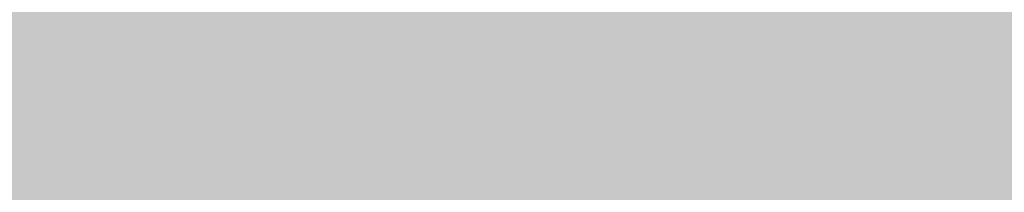
# Model space of a CAD drawing. Units: inches. Extents: x 2091 to 2899, y 967 to 2217.
# Tile 218 of 256: x 2203.2571 to 2203.4104, y 1152.274 to 1152.3009. Entities that reach past the tile are written whole.
import ezdxf

# ---------------------------------------------------------------- set-up
doc = ezdxf.new("R2010")
doc.units = ezdxf.units.IN
doc.layers.add('A-WALL-PATT', color=141, linetype='Continuous', lineweight=13, true_color=0xadddf7)

msp = doc.modelspace()

# ---------------------------------------------------------------- hatches: boundary and pattern name
at = {"layer": 'A-WALL-PATT'}
h = msp.add_hatch(color=256, dxfattribs=at)
h.dxf.hatch_style = 1
h.paths.add_polyline_path([(2803.1436, 2050.91906), (2203.1436, 2050.91906), (2203.1436, 1090.91906), (2803.1436, 1090.91906)])
h.paths.add_polyline_path([(2635.79885, 1147.54046), (2674.52405, 1147.54046, 0.376086), (2678.52967, 1152.8802), (2678.52967, 1159.55647, 0.333335), (2674.52432, 1163.56185), (2674.52432, 1163.56185), (2674.52432, 1192.93439), (2635.80597, 1192.93439), (2597.08762, 1192.93439), (2597.08762, 1163.56185, 0.333335), (2593.08228, 1159.55647), (2593.08228, 1152.8802, 0.376086), (2597.08789, 1147.54046)], flags=0)
h.paths.add_polyline_path([(2436.01043, 1278.24078, 0.000483), (2435.95264, 1278.21503, -0.001328), (2435.93563, 1278.11169, -0.001711), (2436.11644, 1278.04076, 0.002185)], flags=0)
h.paths.add_polyline_path([(2794.1436, 1143.41906), (2794.1436, 1347.41906), (2543.37017, 1347.41906), (2543.37017, 1351.91906), (2794.1436, 1351.91906), (2794.1436, 1392.71355), (2793.9474, 1392.71355), (2793.9474, 1473.5369), (2794.1436, 1473.5369), (2794.1436, 1531.91906), (2650.1436, 1531.91906), (2650.1436, 1536.41906), (2794.1436, 1536.41906), (2794.1436, 1692.41906), (2609.37561, 1692.41906), (2609.37561, 1644.41906), (2604.87561, 1644.41906), (2604.87561, 1744.91906), (2609.37561, 1744.91906), (2609.37561, 1696.91906), (2794.1436, 1696.91906), (2794.1436, 1780.91906), (2609.6436, 1780.91906), (2493.87561, 1780.91906), (2493.87561, 1785.41906), (2609.6436, 1785.41906), (2794.1436, 1785.41906), (2794.1436, 1847.93882), (2793.95122, 1847.93882), (2793.95122, 1928.76217), (2794.1436, 1928.76217), (2794.1436, 1941.41906), (2614.1436, 1941.41906), (2614.1436, 1821.41906), (2609.6436, 1821.41906), (2609.6436, 1941.41906), (2392.1436, 1941.41906), (2392.1436, 1819.91906), (2387.6436, 1819.91906), (2387.6436, 1941.41906), (2212.1436, 1941.41906), (2212.1436, 1783.91906), (2392.1436, 1783.91906), (2392.1436, 1780.91906), (2212.1436, 1780.91906), (2212.1436, 1629.41906), (2387.6436, 1629.41906), (2387.6436, 1744.91906), (2392.1436, 1744.91906), (2392.1436, 1627.91906), (2317.1436, 1627.91906), (2317.1436, 1551.41906), (2317.1436, 1536.41906), (2459.38359, 1536.41906), (2459.38359, 1602.39648), (2463.88359, 1602.39648), (2463.88359, 1531.91906), (2456.6436, 1531.91906), (2456.6436, 1529.91906), (2452.1436, 1529.91906), (2452.1436, 1531.91906), (2312.6436, 1531.91906), (2312.6436, 1551.41906), (2306.1436, 1551.41906), (2306.1436, 1555.91906), (2308.1436, 1555.91906), (2308.1436, 1551.41906), (2312.6436, 1551.41906), (2312.6436, 1627.91906), (2212.1436, 1627.91906), (2212.1436, 1555.91906), (2270.1436, 1555.91906), (2270.1436, 1551.41906), (2212.1436, 1551.41906), (2212.1436, 1351.91906), (2272.1436, 1351.91906), (2272.1436, 1347.41906), (2212.1436, 1347.41906), (2212.1436, 1275.41906), (2308.1436, 1275.41906), (2308.1436, 1351.91906), (2452.1436, 1351.91906), (2452.1436, 1493.91906), (2456.6436, 1493.91906), (2456.6436, 1347.41906), (2312.6436, 1347.41906), (2312.6436, 1270.91906), (2212.1436, 1270.91906), (2212.1436, 1099.91906), (2281.23752, 1099.91906), (2282.87104, 1110.9138), (2282.00834, 1116.9966), (2278.55774, 1121.4204), (2268.20564, 1128.0562), (2272.08764, 1128.0562), (2273.81294, 1131.927), (2279.42034, 1134.6919), (2285.02784, 1135.2449), (2287.61584, 1137.4568), (2288.04714, 1138.0098), (2289.34114, 1140.7747), (2291.06654, 1139.6687), (2292.36054, 1135.2449), (2295.37984, 1136.9038), (2296.24254, 1135.7979), (2297.10524, 1133.033), (2300.12464, 1138.0098), (2303.14394, 1138.0098), (2304.43794, 1135.7979), (2303.14394, 1133.586), (2306.59464, 1134.6919), (2307.88874, 1133.033), (2310.90804, 1135.2449), (2313.92744, 1134.1389), (2315.62686, 1132.4271), (2308.32004, 1117.5496), (2290.20384, 1109.8079), (2288.90984, 1103.1721), (2289.27231, 1099.91906), (2434.91823, 1099.91906), (2431.59323, 1124.78806), (2429.93023, 1169.55306), (2430.92718, 1240.51969), (2435.65893, 1238.18613), (2437.13523, 1196.55406), (2438.79823, 1143.97306), (2442.67823, 1111.99806), (2446.55823, 1099.91906), (2794.1436, 1099.91906), (2794.1436, 1138.91906), (2548.03245, 1138.91906), (2548.03245, 1143.41906), (2548.03245, 1148.81906), (2546.66846, 1148.03156), (2528.68569, 1179.17862, 0.256256), (2512.03245, 1148.81906), (2512.03245, 1143.41906), (2512.03245, 1138.91906), (2507.53245, 1138.91906), (2507.53245, 1143.41906), (2507.53245, 1148.81906, 0.256256), (2490.8792, 1179.17862), (2472.89644, 1148.03156), (2471.53245, 1148.81906), (2471.53245, 1143.41906), (2467.03245, 1143.41906), (2467.03245, 1269.94579, 0.039061), (2460.90999, 1273.58006), (2467.03245, 1273.58006), (2467.03245, 1286.32536, 0.014511), (2465.21619, 1286.76191), (2467.03245, 1287.05258), (2467.03245, 1323.41906), (2471.53245, 1323.41906), (2471.53245, 1148.81906), (2489.53245, 1179.99597), (2490.89644, 1179.20847), (2490.8792, 1179.17862, -0.256256), (2507.53245, 1148.81906), (2507.53245, 1143.41906), (2512.03245, 1143.41906), (2512.03245, 1148.81906, -0.256256), (2528.68569, 1179.17862), (2528.66846, 1179.20847), (2530.03245, 1179.99597), (2548.03245, 1148.81906), (2548.03245, 1143.41906)], flags=16)
h.paths.add_polyline_path([(2607.76855, 1200.94508), (2607.76855, 1265.03063), (2597.08762, 1281.05201), (2619.78459, 1281.05201), (2627.79528, 1337.12686), (2635.79885, 1337.12686), (2643.81666, 1337.12686), (2651.82736, 1281.05201), (2674.52432, 1281.05201), (2663.8434, 1265.03063), (2663.8434, 1200.94508), (2635.80597, 1200.94508)], flags=0)
edge = h.paths.add_edge_path(flags=0)
edge.add_ellipse((13303.89622, 1272.99872), major_axis=(-10595.31304, 0), ratio=0.84230387009, start_angle=0.628237219, end_angle=0.6465541, ccw=False)
edge.add_ellipse((2711.70045, 1156.85268), major_axis=(2.21977, 0), ratio=0.8423039, start_angle=111.53524, end_angle=180.62824, ccw=False)
edge.add_ellipse((13303.15629, 1272.99872), major_axis=(-10593.02631, 0), ratio=0.84230386954, start_angle=0.528271472, end_angle=0.646554097, ccw=False)
edge.add_line((2710.7646, 1175.3333), (2710.12999, 1175.3333))
edge.add_ellipse((2710.12999, 1176.57978), major_axis=(1.47985, 0), ratio=0.8423039, start_angle=180, end_angle=270, ccw=False)
edge.add_line((2708.65014, 1176.57978), (2708.65014, 1200.78291))
edge.add_ellipse((2710.12999, 1200.78291), major_axis=(1.47985, 0), ratio=0.8423039, start_angle=90, end_angle=180, ccw=False)
edge.add_line((2710.12999, 1202.02939), (2710.46508, 1202.02939))
edge.add_ellipse((13303.15629, 1272.99872), major_axis=(-10593.02631, 0), ratio=0.84230386954, start_angle=-0.090229089, end_angle=0.383866779, ccw=False)
edge.add_ellipse((2710.12999, 1290.92703), major_axis=(-1.47985, 0), ratio=0.8423039, start_angle=0, end_angle=90, ccw=False)
edge.add_line((2708.65014, 1290.92703), (2708.65014, 1315.13017))
edge.add_ellipse((2710.12999, 1315.13017), major_axis=(-1.47985, 0), ratio=0.8423039, start_angle=-90, end_angle=0, ccw=False)
edge.add_line((2710.12999, 1316.37665), (2710.70631, 1316.37665))
edge.add_ellipse((3238.40172, 1296.28957), major_axis=(528.234, 0), ratio=0.84230387, start_angle=176.3495724, end_angle=177.8200497, ccw=False)
edge.add_ellipse((2775.06304, 1071.4507), major_axis=(313.30776, 0), ratio=0.84230387, start_angle=102.1259656, end_angle=103.780529, ccw=False)
edge.add_ellipse((2775.06304, 1078.3057), major_axis=(-305.30289, 0), ratio=0.84230387, start_angle=-79.790461, end_angle=-77.5553727, ccw=False)
edge.add_ellipse((2695.14177, 1541.97538), major_axis=(-250.96022, 0), ratio=0.84230387, start_angle=99.256566, end_angle=102.5549326)
edge.add_line((2741.41033, 1334.21426), (2747.13255, 1337.37848))
edge.add_ellipse((2747.53862, 1336.85748), major_axis=(-0.73992, 0), ratio=0.842304, start_angle=270, end_angle=307.93313, ccw=False)
edge.add_ellipse((2747.53862, 1336.85748), major_axis=(-0.73992, 0), ratio=0.842304, start_angle=232.06687, end_angle=270, ccw=False)
edge.add_line((2747.94469, 1337.37848), (2753.66691, 1334.21426))
edge.add_ellipse((2799.93547, 1541.97538), major_axis=(250.96022, 0), ratio=0.84230387, start_angle=257.4450674, end_angle=260.743434)
edge.add_ellipse((2720.01419, 1078.3057), major_axis=(305.30289, 0), ratio=0.84230387, start_angle=77.5553727, end_angle=79.790461, ccw=False)
edge.add_ellipse((2720.01419, 1071.4507), major_axis=(-313.30776, 0), ratio=0.84230387, start_angle=256.219471, end_angle=257.8740344, ccw=False)
edge.add_ellipse((2256.67551, 1296.28957), major_axis=(-528.234, 0), ratio=0.84230387, start_angle=182.1799503, end_angle=183.6504276, ccw=False)
edge.add_line((2784.37092, 1316.37665), (2784.94725, 1316.37665))
edge.add_ellipse((2784.94725, 1315.13017), major_axis=(1.47985, 0), ratio=0.8423039, start_angle=0, end_angle=90, ccw=False)
edge.add_line((2786.42709, 1315.13017), (2786.42709, 1290.92703))
edge.add_ellipse((2784.94725, 1290.92703), major_axis=(1.47985, 0), ratio=0.8423039, start_angle=270, end_angle=360, ccw=False)
edge.add_ellipse((-7808.07906, 1272.99872), major_axis=(10593.02631, 0), ratio=0.84230386954, start_angle=-0.383866779, end_angle=0.090229089, ccw=False)
edge.add_line((2784.61216, 1202.02939), (2784.94725, 1202.02939))
edge.add_ellipse((2784.94725, 1200.78291), major_axis=(1.47985, 0), ratio=0.8423039, start_angle=0, end_angle=90, ccw=False)
edge.add_line((2786.42709, 1200.78291), (2786.42709, 1176.57978))
edge.add_ellipse((2784.94725, 1176.57978), major_axis=(-1.47985, 0), ratio=0.8423039, start_angle=90, end_angle=180, ccw=False)
edge.add_line((2784.94725, 1175.3333), (2784.31264, 1175.3333))
edge.add_ellipse((-7808.07906, 1272.99872), major_axis=(10593.02631, 0), ratio=0.84230386954, start_angle=-0.618643196, end_angle=-0.528271472, ccw=False)
edge.add_ellipse((2783.37678, 1156.85268), major_axis=(-2.21977, 0), ratio=0.8423039, start_angle=179.37176, end_angle=248.46476, ccw=False)
edge.add_ellipse((-7808.81898, 1272.99872), major_axis=(-10595.31304, 0), ratio=0.84230386576, start_angle=179.353445923, end_angle=179.371762803, ccw=False)
edge.add_ellipse((2780.2973, 1153.50079), major_axis=(-5.24643, 0), ratio=0.8423039, start_angle=90, end_angle=179.35345, ccw=False)
edge.add_line((2780.2973, 1149.08171), (2714.77993, 1149.08171))
edge.add_ellipse((2714.77993, 1153.50079), major_axis=(5.24643, 0), ratio=0.8423039, start_angle=180.64655, end_angle=270, ccw=False)
edge = h.paths.add_edge_path(flags=0)
edge.add_line((2718.18737, 1151.00783), (2718.18737, 1170.47236))
edge.add_ellipse((2721.14706, 1170.47236), major_axis=(-2.95969, 0), ratio=0.8423039, start_angle=-90, end_angle=0, ccw=False)
edge.add_line((2721.14706, 1172.96532), (2773.93017, 1172.96532))
edge.add_ellipse((2773.93017, 1170.47236), major_axis=(-2.95969, 0), ratio=0.8423039, start_angle=180, end_angle=270, ccw=False)
edge.add_line((2776.88987, 1170.47236), (2776.88987, 1151.00783))
edge.add_line((2776.88987, 1151.00783), (2718.18737, 1151.00783))
edge = h.paths.add_edge_path(flags=0)
edge.add_line((2718.18737, 1180.23415), (2718.18737, 1199.05783))
edge.add_ellipse((2747.53862, 1320.39864), major_axis=(147.01792, 0), ratio=0.84230387, start_angle=256.4018653, end_angle=283.5981347)
edge.add_line((2776.88987, 1199.05783), (2776.88987, 1180.23415))
edge.add_ellipse((2747.53862, 1301.57496), major_axis=(147.01792, 0), ratio=0.84230387, start_angle=256.4018653, end_angle=283.5981347, ccw=False)
edge = h.paths.add_edge_path(flags=0)
edge.add_ellipse((13303.15629, 1272.99872), major_axis=(-10591.54646, 0), ratio=0.84230386955, start_angle=0.055594314, end_angle=0.377764194, ccw=False)
edge.add_line((2711.61686, 1262.72171), (2715.66741, 1249.4954))
edge.add_ellipse((6413.89196, 1241.69192), major_axis=(-3698.23616, 0), ratio=0.8423038695, start_angle=-0.12089737, end_angle=0.36407635)
edge.add_line((2715.76104, 1218.19245), (2711.93431, 1203.16736))
edge = h.paths.add_edge_path(flags=0)
edge.add_line((2718.18737, 1251.07457), (2716.00249, 1267.45044))
edge.add_ellipse((2742.15117, 1202.18954), major_axis=(81.77258, 0), ratio=0.84230387, start_angle=94.277421, end_angle=111.8349538, ccw=False)
edge.add_line((2737.00975, 1270.93063), (2758.06748, 1270.93063))
edge.add_ellipse((2752.92606, 1202.18954), major_axis=(81.77258, 0), ratio=0.84230387, start_angle=68.1650462, end_angle=85.722579, ccw=False)
edge.add_line((2779.07475, 1267.45044), (2776.88987, 1251.07457))
edge.add_ellipse((2750.33806, 1187.88536), major_axis=(79.57966, 0), ratio=0.84230387, start_angle=67.2080851, end_angle=85.1299304)
edge.add_line((2756.03466, 1254.74366), (2739.04258, 1254.74366))
edge.add_ellipse((2744.73917, 1187.88536), major_axis=(79.57966, 0), ratio=0.84230387, start_angle=94.8700696, end_angle=112.7919149)
edge = h.paths.add_edge_path(flags=0)
edge.add_line((2783.14293, 1203.16736), (2779.31619, 1218.19245))
edge.add_ellipse((-918.81473, 1241.69192), major_axis=(3698.23616, 0), ratio=0.8423038695, start_angle=-0.36407635, end_angle=0.12089737)
edge.add_line((2779.40983, 1249.4954), (2783.46037, 1262.72171))
edge.add_ellipse((-7808.07906, 1272.99872), major_axis=(-10591.54646, 0), ratio=0.84230386954, start_angle=179.622235806, end_angle=179.944405687, ccw=False)
edge = h.paths.add_edge_path(flags=0)
edge.add_ellipse((2734.20089, 1286.69044), major_axis=(-0.35661, 6.34008), ratio=0.6038336, start_angle=89.002014, end_angle=253.657408, ccw=False)
edge.add_line((2730.369, 1286.54181), (2730.369, 1301.35198))
edge.add_line((2730.369, 1301.35198), (2735.91331, 1305.2148))
edge.add_ellipse((2736.38492, 1304.73456), major_axis=(0.73992, 0), ratio=0.842304, start_angle=90, end_angle=134.48021, ccw=False)
edge.add_line((2736.38492, 1305.3578), (2738.03278, 1305.3578))
edge.add_line((2738.03278, 1305.3578), (2738.03278, 1307.70793))
edge.add_ellipse((2794.20164, 1307.70793), major_axis=(56.16886, 0), ratio=0.84230387, start_angle=150.56143, end_angle=180, ccw=False)
edge.add_ellipse((2700.87559, 1307.70793), major_axis=(-56.16886, 0), ratio=0.84230387, start_angle=180, end_angle=209.43857, ccw=False)
edge.add_line((2757.04445, 1307.70793), (2757.04445, 1305.3578))
edge.add_line((2757.04445, 1305.3578), (2758.69232, 1305.3578))
edge.add_ellipse((2758.69232, 1304.73456), major_axis=(-0.73992, 0), ratio=0.842304, start_angle=225.51979, end_angle=270, ccw=False)
edge.add_line((2759.16392, 1305.2148), (2764.70823, 1301.35198))
edge.add_line((2764.70823, 1301.35198), (2764.70823, 1286.54181))
edge.add_ellipse((2760.87634, 1286.69044), major_axis=(0.35661, 6.34008), ratio=0.6038336, start_angle=106.342592, end_angle=270.997986, ccw=False)
edge.add_line((2757.04445, 1285.79709), (2757.04445, 1307.70793))
edge.add_ellipse((2700.87559, 1307.70793), major_axis=(-56.16886, 0), ratio=0.84230387, start_angle=180, end_angle=209.43857)
edge.add_ellipse((2794.20164, 1307.70793), major_axis=(56.16886, 0), ratio=0.84230387, start_angle=150.56143, end_angle=180)
edge.add_line((2738.03278, 1307.70793), (2738.03278, 1285.79709))
h.paths.add_polyline_path([(2417.81227, 1104.4497), (2413.49227, 1102.5297), (2410.61227, 1103.9697), (2409.17227, 1106.3697), (2407.25227, 1107.3297), (2406.29227, 1109.7297), (2405.33227, 1114.0497), (2405.33227, 1117.8897), (2406.29227, 1120.1297), (2407.25227, 1119.8097), (2408.84832, 1118.32766), (2410.17395, 1119.42417), (2410.21127, 1120.4057), (2411.04073, 1121.41905), (2410.69927, 1119.8587), (2410.17395, 1119.42417), (2410.08845, 1117.17611), (2411.13284, 1116.20632), (2413.97227, 1119.3297), (2416.85227, 1120.7697), (2416.86972, 1120.79878), (2417.03507, 1119.40512), (2417.89621, 1118.14338), (2418.29227, 1118.3697), (2419.54445, 1120.03927), (2419.36092, 1118.38749), (2419.03211, 1119.35615), (2418.39894, 1118.51193), (2419.25227, 1114.5297), (2418.79409, 1107.19879)], flags=0)
h.paths.add_polyline_path([(2508.87017, 1347.41906), (2508.37017, 1347.41906), (2508.37017, 1351.91906), (2508.87017, 1351.91906)], flags=0)
h.paths.add_polyline_path([(2473.37017, 1347.41906), (2472.37017, 1347.41906), (2467.87017, 1347.41906), (2467.87017, 1455.41906), (2472.37017, 1455.41906), (2472.37017, 1352.41906), (2473.37017, 1352.41906)], flags=0)
h.paths.add_polyline_path([(2352.10624, 1217.4462), (2349.22624, 1218.8862), (2347.78624, 1221.2862), (2345.86624, 1222.2462), (2344.90624, 1224.6462), (2343.94624, 1228.9662), (2343.94624, 1232.8062), (2344.90624, 1235.0462), (2345.86624, 1234.7262), (2347.46229, 1233.24415), (2348.78792, 1234.34066), (2348.82524, 1235.3222), (2349.6547, 1236.33555), (2349.31324, 1234.7752), (2348.78792, 1234.34066), (2348.70242, 1232.0926), (2349.74681, 1231.12282), (2352.58624, 1234.2462), (2355.46624, 1235.6862), (2355.48369, 1235.71528), (2355.64904, 1234.32161), (2356.51018, 1233.05988), (2356.90624, 1233.2862), (2358.15842, 1234.95576), (2357.97489, 1233.30398), (2357.64608, 1234.27264), (2357.01291, 1233.42842), (2357.86624, 1229.4462), (2357.40806, 1222.11529), (2356.42624, 1219.3662)], flags=0)
h.paths.add_polyline_path([(2348.2968, 1112.22442), (2347.0138, 1112.31042), (2345.5298, 1114.12742), (2345.7318, 1115.85842), (2346.8118, 1116.98242), (2346.8118, 1114.64642), (2345.8668, 1114.21442), (2346.8798, 1114.30042)], flags=0)
h.paths.add_polyline_path([(2347.0138, 1110.92642), (2346.2718, 1110.49342), (2346.6098, 1111.18642)], flags=0)
h.paths.add_polyline_path([(2345.8668, 1118.19442), (2345.5298, 1117.32942), (2343.7078, 1118.02142), (2344.3828, 1118.62642)], flags=0)
h.paths.add_polyline_path([(2346.6768, 1109.28242), (2346.0698, 1108.07142), (2345.8668, 1110.06142)], flags=0)
h.paths.add_polyline_path([(2345.0568, 1119.75142), (2343.6398, 1119.75142), (2343.9778, 1121.13542)], flags=0)
h.paths.add_polyline_path([(2345.2598, 1116.55042), (2345.1248, 1115.85842), (2344.9218, 1115.68542), (2344.7198, 1116.37742)], flags=0)
h.paths.add_polyline_path([(2345.6648, 1112.31042), (2345.4618, 1111.53242), (2344.0448, 1111.96442), (2344.6518, 1112.57042)], flags=0)
h.paths.add_polyline_path([(2345.1918, 1113.34942), (2344.4498, 1113.86842), (2344.7198, 1114.38742)], flags=0)
h.paths.add_polyline_path([(2344.6518, 1116.80942), (2344.1798, 1115.68542), (2344.6518, 1115.33942), (2343.9098, 1114.90642), (2343.0328, 1115.94442), (2343.6398, 1116.46342)], flags=0)
h.paths.add_polyline_path([(2345.8668, 1106.68642), (2344.9898, 1105.56242), (2344.5168, 1106.60042)], flags=0)
h.paths.add_polyline_path([(2344.8548, 1110.06142), (2344.5168, 1109.28242), (2344.1128, 1109.71542)], flags=0)
h.paths.add_polyline_path([(2344.0448, 1113.52242), (2343.4378, 1113.08942), (2342.7628, 1113.95442)], flags=0)
h.paths.add_polyline_path([(2344.3148, 1111.01242), (2342.9648, 1110.32042), (2342.9648, 1111.09942)], flags=0)
h.paths.add_polyline_path([(2345.1248, 1104.69742), (2344.5848, 1103.74542), (2344.4498, 1104.26442)], flags=0)
h.paths.add_polyline_path([(2342.8298, 1121.22242), (2341.7498, 1120.53042), (2340.5358, 1121.04942), (2340.1308, 1121.82842), (2340.6708, 1122.95242), (2341.1428, 1121.82842), (2341.6148, 1122.00142)], flags=0)
h.paths.add_polyline_path([(2342.9648, 1119.75142), (2343.0328, 1118.45342), (2342.0878, 1118.02142), (2342.0198, 1119.49142)], flags=0)
h.paths.add_polyline_path([(2342.6948, 1116.89642), (2341.9528, 1116.63642), (2342.0198, 1117.32942)], flags=0)
h.paths.add_polyline_path([(2343.0328, 1112.22442), (2342.0198, 1111.79142), (2341.5478, 1112.22442), (2342.3578, 1113.34942)], flags=0)
h.paths.add_polyline_path([(2343.7748, 1104.43742), (2342.6278, 1102.88042), (2342.6948, 1104.61042), (2343.4378, 1105.12942)], flags=0)
h.paths.add_polyline_path([(2342.0198, 1115.07942), (2340.8058, 1115.51242), (2340.9408, 1116.37742)], flags=0)
h.paths.add_polyline_path([(2341.4808, 1120.09742), (2341.4808, 1119.40542), (2341.0758, 1119.57842), (2341.1428, 1120.09742)], flags=0)
h.paths.add_polyline_path([(2341.8178, 1114.47342), (2340.9408, 1113.08942), (2340.8058, 1114.56042)], flags=0)
h.paths.add_polyline_path([(2341.1428, 1118.54042), (2340.9408, 1116.98242), (2339.0508, 1117.67542), (2339.0508, 1118.62642)], flags=0)
h.paths.add_polyline_path([(2342.6948, 1101.66842), (2341.9528, 1101.84142), (2342.5598, 1102.36142)], flags=0)
h.paths.add_polyline_path([(2340.3328, 1119.66542), (2338.4438, 1119.57842), (2337.9038, 1120.35742), (2339.6578, 1120.61642)], flags=0)
h.paths.add_polyline_path([(2340.3328, 1115.33942), (2340.0628, 1113.69542), (2339.3878, 1115.33942)], flags=0)
h.paths.add_polyline_path([(2341.8178, 1103.83142), (2341.5478, 1102.88042), (2341.1428, 1103.65842)], flags=0)
h.paths.add_polyline_path([(2339.0508, 1122.86642), (2337.2958, 1121.82842), (2337.0938, 1123.12542), (2337.7688, 1123.81842)], flags=0)
h.paths.add_polyline_path([(2339.1178, 1121.74142), (2338.8478, 1121.22242), (2338.1738, 1121.04942), (2338.3758, 1121.56842)], flags=0)
h.paths.add_polyline_path([(2339.1858, 1119.31942), (2338.6458, 1118.71342), (2338.2408, 1118.10742), (2338.2408, 1118.88642)], flags=0)
h.paths.add_polyline_path([(2341.1428, 1101.92842), (2340.6028, 1101.23642), (2340.0628, 1101.84142), (2340.6028, 1102.36142)], flags=0)
h.paths.add_polyline_path([(2337.6338, 1117.76142), (2336.6208, 1118.28042), (2337.2958, 1118.97242)], flags=0)
h.paths.add_polyline_path([(2336.8238, 1119.57842), (2334.7988, 1118.97242), (2335.2038, 1120.35742), (2336.5538, 1120.87642)], flags=0)
h.paths.add_polyline_path([(2339.1178, 1100.45742), (2337.3638, 1100.54342), (2336.7558, 1101.23642)], flags=0)
h.paths.add_polyline_path([(2336.3508, 1122.43342), (2336.0138, 1121.91442), (2334.9338, 1122.43342), (2334.5288, 1123.47142), (2335.7438, 1122.77942)], flags=0)
h.paths.add_polyline_path([(2334.7318, 1120.87642), (2334.2588, 1120.35742), (2334.0568, 1120.78942), (2334.5968, 1121.30842)], flags=0)
h.paths.add_polyline_path([(2334.4618, 1122.17442), (2332.5718, 1121.30842), (2331.3568, 1122.17442), (2332.0998, 1122.86642)], flags=0)
h.paths.add_polyline_path([(2334.2588, 1118.54042), (2333.3818, 1118.45342), (2333.6518, 1119.31942)], flags=0)
h.paths.add_polyline_path([(2335.5418, 1102.27442), (2334.1918, 1102.62042), (2335.2718, 1103.31242)], flags=0)
h.paths.add_polyline_path([(2332.7068, 1119.66542), (2331.6948, 1120.44342), (2332.5048, 1120.78942)], flags=0)
h.paths.add_polyline_path([(2334.7318, 1101.14942), (2333.5168, 1101.58242), (2333.9888, 1101.75542)], flags=0)
h.paths.add_polyline_path([(2332.6398, 1116.63642), (2331.0868, 1116.29042), (2331.9648, 1118.19442)], flags=0)
h.paths.add_polyline_path([(2330.7498, 1121.56842), (2330.2768, 1120.27042), (2328.5228, 1119.31942), (2328.9948, 1121.04942)], flags=0)
h.paths.add_polyline_path([(2330.7498, 1118.62642), (2330.0078, 1117.50242), (2329.8728, 1118.02142)], flags=0)
h.paths.add_polyline_path([(2332.0998, 1102.36142), (2330.5468, 1102.01442), (2331.6948, 1102.96642)], flags=0)
h.paths.add_polyline_path([(2329.5348, 1113.60842), (2329.0628, 1112.31042), (2328.5898, 1113.34942)], flags=0)
h.paths.add_polyline_path([(2328.3878, 1117.84842), (2327.5098, 1116.55042), (2327.1728, 1117.76142)], flags=0)
h.paths.add_polyline_path([(2329.7378, 1106.51342), (2329.5348, 1105.30242), (2328.2528, 1106.08142)], flags=0)
h.paths.add_polyline_path([(2328.6578, 1114.38742), (2328.0498, 1114.12742), (2328.3198, 1114.90642)], flags=0)
h.paths.add_polyline_path([(2328.3198, 1112.22442), (2327.1058, 1112.13742), (2326.7008, 1112.65642)], flags=0)
h.paths.add_polyline_path([(2326.9028, 1115.25242), (2326.7008, 1114.12742), (2325.2158, 1113.60842), (2326.0928, 1115.33942)], flags=0)
h.paths.add_polyline_path([(2326.6328, 1108.33042), (2326.0928, 1107.37942), (2325.8908, 1108.50342), (2326.4978, 1109.10942)], flags=0)
h.paths.add_polyline_path([(2615.1436, 1531.91906), (2609.6436, 1531.91906), (2609.6436, 1620.41906), (2614.1436, 1620.41906), (2614.1436, 1536.41906), (2615.1436, 1536.41906)], flags=0)
h.paths.add_polyline_path([(2545.1436, 1563.41906), (2464.1436, 1563.41906), (2464.1436, 1632.41906), (2509.1436, 1632.41906), (2509.1436, 1627.91906), (2509.1436, 1603.91906), (2468.6436, 1603.91906), (2468.6436, 1567.91906), (2540.6436, 1567.91906), (2540.6436, 1591.91906), (2545.1436, 1591.91906)], flags=0)
h.paths.add_polyline_path([(2388.96905, 1549.98573), (2357.43418, 1549.98573), (2357.43418, 1623.36078), (2399.36278, 1623.36078), (2435.68947, 1623.36078), (2435.59255, 1602.55927), (2435.59255, 1602.39648), (2388.96905, 1602.39648)], flags=0)
h.paths.add_polyline_path([(2388.88063, 1555.80915), (2374.90443, 1555.80915), (2374.90443, 1600.57156), (2374.90443, 1615.45765), (2406.35088, 1615.45765), (2406.35088, 1618.93943), (2412.17429, 1615.45765), (2406.35088, 1611.97586), (2406.35088, 1615.45765), (2388.88063, 1615.45765)], flags=0)
h.paths.add_polyline_path([(2568.87561, 1644.41906), (2453.37561, 1644.41906), (2453.37561, 1785.41906), (2457.87561, 1785.41906), (2457.87561, 1648.91906), (2568.87561, 1648.91906)], flags=0)
h.paths.add_polyline_path([(2212.1436, 1945.91906), (2212.1436, 2041.91906), (2794.1436, 2041.91906), (2794.1436, 1945.91906)], flags=16)
h.paths.add_polyline_path([(2271.08273, 1964.31724), (2776.85297, 1964.31724), (2776.85297, 2037.16962), (2271.08273, 2037.16962)], flags=8)
h.paths.add_polyline_path([(2380.64929, 1536.82414), (2461.04081, 1536.82414), (2461.04081, 1554.65259), (2380.64929, 1554.65259)], flags=8)
h.paths.add_polyline_path([(2240.75571, 1609.72545), (2309.18583, 1609.72545), (2309.18583, 1617.6982), (2240.75571, 1617.6982)], flags=8)
h.paths.add_polyline_path([(2212.67726, 1313.5041), (2282.59152, 1313.5041), (2282.59152, 1322.74524), (2212.67726, 1322.74524)], flags=8)
h.paths.add_polyline_path([(2457.11198, 1114.77857), (2558.48158, 1114.77857), (2558.48158, 1142.21968), (2457.11198, 1142.21968)], flags=8)
h.paths.add_polyline_path([(2473.44234, 1273.01007), (2604.64123, 1273.01007), (2604.64123, 1318.34693), (2473.44234, 1318.34693)], flags=8)
h.paths.add_polyline_path([(2638.8763, 1626.97743), (2684.25037, 1627.97674), (2684.03848, 1637.59749), (2638.66442, 1636.59819)], flags=8)
h.paths.add_polyline_path([(2537.59055, 1453.79345), (2628.38955, 1453.79345), (2628.38955, 1475.34481), (2537.59055, 1475.34481)], flags=8)
h.paths.add_polyline_path([(2504.13764, 1714.6324), (2554.64719, 1714.6324), (2554.64719, 1730.23771), (2504.13764, 1730.23771)], flags=8)
h.paths.add_polyline_path([(2487.50118, 1575.65187), (2535.09712, 1575.65187), (2535.09712, 1598.37765), (2487.50118, 1598.37765)], flags=8)
h.paths.add_polyline_path([(2709.0994, 1735.71028), (2740.0166, 1735.71028), (2740.0166, 1749.93764), (2709.0994, 1749.93764)], flags=8)
h.paths.add_polyline_path([(2442.43842, 1792.17166), (2564.72884, 1792.17166), (2564.72884, 1842.00016), (2442.43842, 1842.00016)], flags=8)
h.paths.add_polyline_path([(2655.8158, 1809.64408), (2789.52014, 1806.6938), (2790.08498, 1832.29164), (2656.38064, 1835.24192)], flags=8)
h.paths.add_polyline_path([(2234.8427, 1797.72014), (2368.59285, 1794.76885), (2369.16072, 1820.50413), (2235.41056, 1823.45542)], flags=8)
h.paths.add_polyline_path([(2245.13847, 1644.00633), (2398.42773, 1640.6239), (2398.99484, 1666.32482), (2245.70557, 1669.70725)], flags=8)
h.paths.add_polyline_path([(2306.14285, 1431.16852), (2413.76831, 1428.79369), (2414.33315, 1454.39153), (2306.70768, 1456.76636)], flags=8)
h.paths.add_polyline_path([(2306.83458, 1458.23314), (2393.38048, 1456.32345), (2393.93281, 1481.35436), (2307.38691, 1483.26405)], flags=8)

doc.saveas('drawing.dxf')
